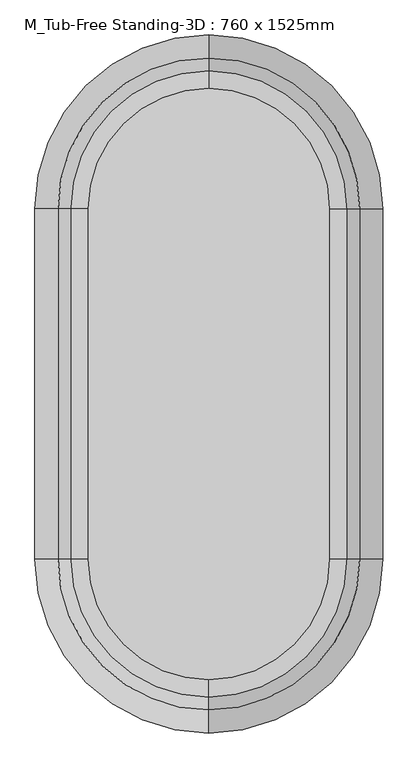
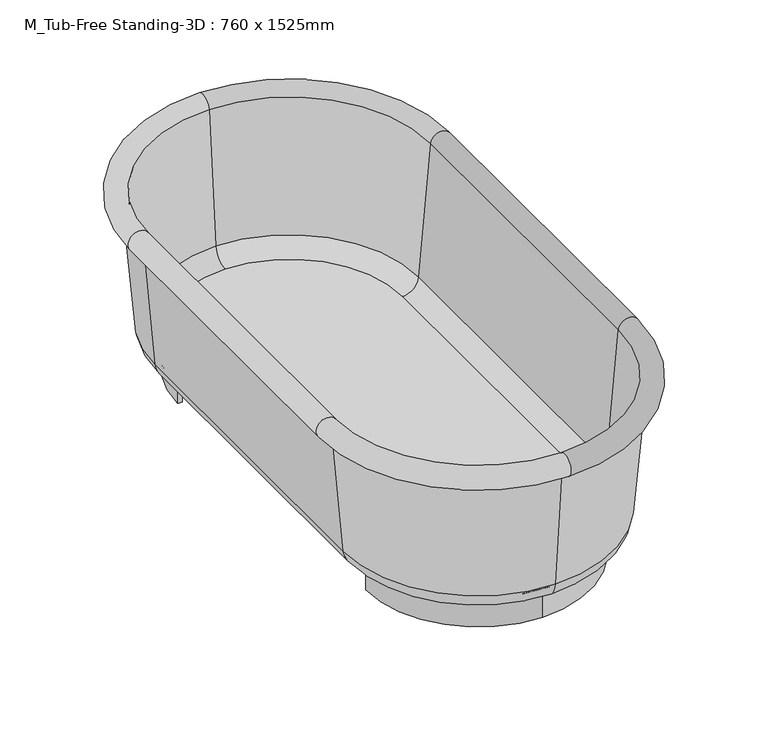
"""IFC4 building model written with IfcOpenShell, lengths in millimetres: flow terminal geometry, M_Tub-Free Standing-3D : 760 x 1525mm."""

from ifc_helpers import new_model, si_unit, point, frame, frame_2d, origin, origin_with_axes, place, context, project, spatial, polyline, circle_curve, ellipse_curve, trimmed, segment, composite_curve, outline, extrude, source, transform, mapped, element, save
from ifc_brep_helpers import plane_surface, cylinder_surface, revolved_surface, advanced_brep


def m_tub_free_standing_3d_760_x_1525mm_d9cb411c(model_context):
    return source(origin(), model_context, "Body", "SolidModel", [
        extrude(outline(composite_curve([segment(trimmed(circle_curve(frame_2d((0.0, -382.5)), 263.2824236), [point((0.0, -645.7824236))], [point((-263.2824236, -382.5))], False, "CARTESIAN"), True, "CONTINUOUS"), segment(polyline([(-263.2824236, -382.5), (-253.0, -382.5)]), True, "CONTINUOUS"), segment(trimmed(circle_curve(frame_2d((0.0, -382.5)), 253.0), [point((-253.0, -382.5))], [point((0.0, -635.5))], True, "CARTESIAN"), True, "CONTINUOUS"), segment(trimmed(circle_curve(frame_2d((0.0, -382.5)), 253.0), [point((0.0, -635.5))], [point((253.0, -382.5))], True, "CARTESIAN"), True, "CONTINUOUS"), segment(polyline([(253.0, -382.5), (263.2824236, -382.5)]), True, "CONTINUOUS"), segment(trimmed(circle_curve(frame_2d((0.0, -382.5)), 263.2824236), [point((263.2824236, -382.5))], [point((0.0, -645.7824236))], False, "CARTESIAN"), True, "CONTINUOUS")], self_intersect=False)), origin_with_axes(), (0.0, 0.0, 1.0), 66.3),
        advanced_brep(
        [(0.0, 635.5, 0.0), (-253.0, 382.5, 0.0), (-263.2824236, 382.5, 0.0), (0.0, 645.7824236, 0.0), (263.2824236, 382.5, 0.0), (253.0, 382.5, 0.0), (253.0, 382.5, 66.3), (0.0, 635.5, 66.3), (263.2824236, 382.5, 65.9536107), (263.2824236, 382.5, 66.3), (0.0, 645.7824236, 65.9536107), (-263.2824236, 382.5, 65.9536107), (-253.0, 382.5, 66.3), (-263.2824236, 382.5, 66.3), (-263.2824236, -382.5, 81.38125), (0.0, -645.7824236, 81.38125), (263.2824236, -382.5, 81.38125), (263.2824236, 382.5, 81.38125), (0.0, 645.7824236, 81.38125), (-263.2824236, 382.5, 81.38125), (263.2824236, -382.5, 66.3), (0.0, -645.7824236, 66.3), (-263.2824236, -382.5, 66.3), (-263.2824236, -382.5, 80.8774627), (0.0, -645.7824236, 80.8774627), (263.2824236, -382.5, 80.8774627), (263.2824236, 382.5, 80.8774627), (0.0, 645.7824236, 80.8774627), (-263.2824236, 382.5, 80.8774627), (0.0, -724.4, 409.2), (341.9, -382.5, 409.2), (354.6, -382.5, 409.2), (0.0, -737.1, 409.2), (0.0, -698.6045038, 114.3561295), (316.1045038, -382.5, 114.3561295), (0.0, -645.7824236, 65.9536107), (263.2824236, -382.5, 65.9536107), (0.0, -683.7374416, 115.6568289), (301.2374416, -382.5, 115.6568289), (0.0, -711.9561556, 438.1982063), (329.4561556, -382.5, 438.1982063), (-354.6, -382.5, 409.2), (-341.9, -382.5, 409.2), (-316.1045038, -382.5, 114.3561295), (-263.2824236, -382.5, 65.9536107), (-301.2374416, -382.5, 115.6568289), (-329.4561556, -382.5, 438.1982063), (-354.6, 382.5, 409.2), (-341.9, 382.5, 409.2), (-316.1045038, 382.5, 114.3561295), (-301.2374416, 382.5, 115.6568289), (-329.4561556, 382.5, 438.1982063), (0.0, 737.1, 409.2), (0.0, 724.4, 409.2), (0.0, 698.6045038, 114.3561295), (0.0, 683.7374416, 115.6568289), (0.0, 711.9561556, 438.1982063), (354.6, 382.5, 409.2), (341.9, 382.5, 409.2), (316.1045038, 382.5, 114.3561295), (301.2374416, 382.5, 115.6568289), (329.4561556, 382.5, 438.1982063)],
        [
            (0, 1, circle_curve(frame((0.0, 382.5, 0.0), z_axis=(0.0, 0.0, 1.0), x_axis=(1.0, 0.0, 0.0)), 253.0)),
            (1, 2),
            (2, 3, circle_curve(frame((0.0, 382.5, 0.0), z_axis=(0.0, 0.0, -1.0), x_axis=(1.0, 0.0, 0.0)), 263.2824236)),
            (3, 4, circle_curve(frame((0.0, 382.5, 0.0), z_axis=(0.0, 0.0, -1.0), x_axis=(1.0, 0.0, 0.0)), 263.2824236)),
            (4, 5),
            (5, 0, circle_curve(frame((0.0, 382.5, 0.0), z_axis=(0.0, 0.0, 1.0), x_axis=(1.0, 0.0, 0.0)), 253.0)),
            (5, 6),
            (6, 7, circle_curve(frame((0.0, 382.5, 66.3), z_axis=(0.0, 0.0, 1.0), x_axis=(1.0, 0.0, 0.0)), 253.0)),
            (7, 0),
            (4, 8),
            (8, 9),
            (9, 6),
            (3, 10),
            (10, 8, circle_curve(frame((0.0, 382.5, 65.9536107), z_axis=(0.0, 0.0, -1.0), x_axis=(1.0, 0.0, 0.0)), 263.2824236)),
            (2, 11),
            (11, 10, circle_curve(frame((0.0, 382.5, 65.9536107), z_axis=(0.0, 0.0, -1.0), x_axis=(1.0, 0.0, 0.0)), 263.2824236)),
            (1, 12),
            (12, 13),
            (13, 11),
            (7, 12, circle_curve(frame((0.0, 382.5, 66.3), z_axis=(0.0, 0.0, 1.0), x_axis=(1.0, 0.0, 0.0)), 253.0)),
            (14, 15, circle_curve(frame((0.0, -382.5, 81.38125), z_axis=(0.0, 0.0, 1.0), x_axis=(0.0, -1.0, 0.0)), 263.2824236)),
            (15, 16, circle_curve(frame((0.0, -382.5, 81.38125), z_axis=(0.0, 0.0, 1.0), x_axis=(0.0, -1.0, 0.0)), 263.2824236)),
            (16, 17),
            (17, 18, circle_curve(frame((0.0, 382.5, 81.38125), z_axis=(0.0, 0.0, 1.0), x_axis=(0.0, -1.0, 0.0)), 263.2824236)),
            (18, 19, circle_curve(frame((0.0, 382.5, 81.38125), z_axis=(0.0, 0.0, 1.0), x_axis=(0.0, -1.0, 0.0)), 263.2824236)),
            (19, 14),
            (9, 20),
            (20, 21, circle_curve(frame((0.0, -382.5, 66.3), z_axis=(0.0, 0.0, -1.0), x_axis=(1.0, 0.0, 0.0)), 263.2824236)),
            (21, 22, circle_curve(frame((0.0, -382.5, 66.3), z_axis=(0.0, 0.0, -1.0), x_axis=(0.0, -1.0, 0.0)), 263.2824236)),
            (22, 13),
            (14, 23),
            (23, 24, circle_curve(frame((0.0, -382.5, 80.8774627), z_axis=(0.0, 0.0, 1.0), x_axis=(0.0, -1.0, 0.0)), 263.2824236)),
            (24, 15),
            (24, 25, circle_curve(frame((0.0, -382.5, 80.8774627), z_axis=(0.0, 0.0, 1.0), x_axis=(0.0, -1.0, 0.0)), 263.2824236)),
            (25, 16),
            (25, 26),
            (26, 17),
            (26, 27, circle_curve(frame((0.0, 382.5, 80.8774627), z_axis=(0.0, 0.0, 1.0), x_axis=(0.0, -1.0, 0.0)), 263.2824236)),
            (27, 18),
            (27, 28, circle_curve(frame((0.0, 382.5, 80.8774627), z_axis=(0.0, 0.0, 1.0), x_axis=(0.0, -1.0, 0.0)), 263.2824236)),
            (28, 19),
            (28, 23),
            (29, 30, circle_curve(frame((0.0, -382.5, 409.2), z_axis=(0.0, 0.0, 1.0), x_axis=(1.0, 0.0, 0.0)), 341.9)),
            (30, 31),
            (31, 32, circle_curve(frame((0.0, -382.5, 409.2), z_axis=(0.0, 0.0, -1.0), x_axis=(1.0, 0.0, 0.0)), 354.6)),
            (32, 29),
            (29, 33),
            (33, 34, circle_curve(frame((0.0, -382.5, 114.3561295), z_axis=(0.0, 0.0, 1.0), x_axis=(1.0, 0.0, 0.0)), 316.1045038)),
            (34, 30),
            (33, 35, circle_curve(frame((0.0, -645.7824236, 118.9774627), z_axis=(1.0, 0.0, 0.0), x_axis=(0.0, -1.0, 0.0)), 53.023852)),
            (35, 36, circle_curve(frame((0.0, -382.5, 65.9536107), z_axis=(0.0, 0.0, 1.0), x_axis=(1.0, 0.0, 0.0)), 263.2824236)),
            (36, 34, circle_curve(frame((263.2824236, -382.5, 118.9774627), z_axis=(0.0, -1.0, 0.0), x_axis=(1.0, 0.0, 0.0)), 53.023852)),
            (35, 21),
            (20, 36),
            (37, 38, circle_curve(frame((0.0, -382.5, 115.6568289), z_axis=(0.0, 0.0, 1.0), x_axis=(1.0, 0.0, 0.0)), 301.2374416)),
            (38, 25, circle_curve(frame((263.2824236, -382.5, 118.9774627), z_axis=(0.0, 1.0, 0.0), x_axis=(1.0, 0.0, 0.0)), 38.1)),
            (24, 37, circle_curve(frame((0.0, -645.7824236, 118.9774627), z_axis=(-1.0, 0.0, 0.0), x_axis=(0.0, -1.0, 0.0)), 38.1)),
            (37, 39),
            (39, 40, circle_curve(frame((0.0, -382.5, 438.1982063), z_axis=(0.0, 0.0, 1.0), x_axis=(1.0, 0.0, 0.0)), 329.4561556)),
            (40, 38),
            (31, 40, circle_curve(frame((354.6, -382.5, 434.6), z_axis=(0.0, -1.0, 0.0), x_axis=(1.0, 0.0, 0.0)), 25.4)),
            (39, 32, circle_curve(frame((0.0, -737.1, 434.6), z_axis=(1.0, 0.0, 0.0), x_axis=(0.0, -1.0, 0.0)), 25.4)),
            (32, 41, circle_curve(frame((0.0, -382.5, 409.2), z_axis=(0.0, 0.0, -1.0), x_axis=(0.0, -1.0, 0.0)), 354.6)),
            (41, 42),
            (42, 29, circle_curve(frame((0.0, -382.5, 409.2), z_axis=(0.0, 0.0, 1.0), x_axis=(0.0, -1.0, 0.0)), 341.9)),
            (42, 43),
            (43, 33, circle_curve(frame((0.0, -382.5, 114.3561295), z_axis=(0.0, 0.0, 1.0), x_axis=(0.0, -1.0, 0.0)), 316.1045038)),
            (43, 44, circle_curve(frame((-263.2824236, -382.5, 118.9774627), z_axis=(0.0, -1.0, 0.0), x_axis=(-1.0, 0.0, 0.0)), 53.023852)),
            (44, 35, circle_curve(frame((0.0, -382.5, 65.9536107), z_axis=(0.0, 0.0, 1.0), x_axis=(0.0, -1.0, 0.0)), 263.2824236)),
            (44, 22),
            (23, 45, circle_curve(frame((-263.2824236, -382.5, 118.9774627), z_axis=(0.0, 1.0, 0.0), x_axis=(-1.0, 0.0, 0.0)), 38.1)),
            (45, 37, circle_curve(frame((0.0, -382.5, 115.6568289), z_axis=(0.0, 0.0, 1.0), x_axis=(0.0, -1.0, 0.0)), 301.2374416)),
            (45, 46),
            (46, 39, circle_curve(frame((0.0, -382.5, 438.1982063), z_axis=(0.0, 0.0, 1.0), x_axis=(0.0, -1.0, 0.0)), 329.4561556)),
            (46, 41, circle_curve(frame((-354.6, -382.5, 434.6), z_axis=(0.0, -1.0, 0.0), x_axis=(-1.0, 0.0, 0.0)), 25.4)),
            (41, 47),
            (47, 48),
            (48, 42),
            (48, 49),
            (49, 43),
            (49, 11, circle_curve(frame((-263.2824236, 382.5, 118.9774627), z_axis=(0.0, -1.0, 0.0), x_axis=(-1.0, 0.0, 0.0)), 53.023852)),
            (11, 44),
            (28, 50, circle_curve(frame((-263.2824236, 382.5, 118.9774627), z_axis=(0.0, 1.0, 0.0), x_axis=(-1.0, 0.0, 0.0)), 38.1)),
            (50, 45),
            (50, 51),
            (51, 46),
            (51, 47, circle_curve(frame((-354.6, 382.5, 434.6), z_axis=(0.0, -1.0, 0.0), x_axis=(-1.0, 0.0, 0.0)), 25.4)),
            (47, 52, circle_curve(frame((0.0, 382.5, 409.2), z_axis=(0.0, 0.0, -1.0), x_axis=(-1.0, 0.0, 0.0)), 354.6)),
            (52, 53),
            (53, 48, circle_curve(frame((0.0, 382.5, 409.2), z_axis=(0.0, 0.0, 1.0), x_axis=(-1.0, 0.0, 0.0)), 341.9)),
            (53, 54),
            (54, 49, circle_curve(frame((0.0, 382.5, 114.3561295), z_axis=(0.0, 0.0, 1.0), x_axis=(-1.0, 0.0, 0.0)), 316.1045038)),
            (54, 10, circle_curve(frame((0.0, 645.7824236, 118.9774627), z_axis=(-1.0, 0.0, 0.0), x_axis=(0.0, 1.0, 0.0)), 53.023852)),
            (27, 55, circle_curve(frame((0.0, 645.7824236, 118.9774627), z_axis=(1.0, 0.0, 0.0), x_axis=(0.0, 1.0, 0.0)), 38.1)),
            (55, 50, circle_curve(frame((0.0, 382.5, 115.6568289), z_axis=(0.0, 0.0, 1.0), x_axis=(-1.0, 0.0, 0.0)), 301.2374416)),
            (55, 56),
            (56, 51, circle_curve(frame((0.0, 382.5, 438.1982063), z_axis=(0.0, 0.0, 1.0), x_axis=(-1.0, 0.0, 0.0)), 329.4561556)),
            (56, 52, circle_curve(frame((0.0, 737.1, 434.6), z_axis=(-1.0, 0.0, 0.0), x_axis=(0.0, 1.0, 0.0)), 25.4)),
            (52, 57, circle_curve(frame((0.0, 382.5, 409.2), z_axis=(0.0, 0.0, -1.0), x_axis=(0.0, 1.0, 0.0)), 354.6)),
            (57, 58),
            (58, 53, circle_curve(frame((0.0, 382.5, 409.2), z_axis=(0.0, 0.0, 1.0), x_axis=(0.0, 1.0, 0.0)), 341.9)),
            (58, 59),
            (59, 54, circle_curve(frame((0.0, 382.5, 114.3561295), z_axis=(0.0, 0.0, 1.0), x_axis=(0.0, 1.0, 0.0)), 316.1045038)),
            (59, 8, circle_curve(frame((263.2824236, 382.5, 118.9774627), z_axis=(0.0, 1.0, 0.0), x_axis=(1.0, 0.0, 0.0)), 53.023852)),
            (26, 60, circle_curve(frame((263.2824236, 382.5, 118.9774627), z_axis=(0.0, -1.0, 0.0), x_axis=(1.0, 0.0, 0.0)), 38.1)),
            (60, 55, circle_curve(frame((0.0, 382.5, 115.6568289), z_axis=(0.0, 0.0, 1.0), x_axis=(0.0, 1.0, 0.0)), 301.2374416)),
            (60, 61),
            (61, 56, circle_curve(frame((0.0, 382.5, 438.1982063), z_axis=(0.0, 0.0, 1.0), x_axis=(0.0, 1.0, 0.0)), 329.4561556)),
            (61, 57, circle_curve(frame((354.6, 382.5, 434.6), z_axis=(0.0, 1.0, 0.0), x_axis=(1.0, 0.0, 0.0)), 25.4)),
            (30, 58),
            (57, 31),
            (34, 59),
            (36, 8),
            (38, 60),
            (40, 61),
        ],
        [
            plane_surface(frame((253.0, 382.5, 0.0), z_axis=(0.0, 0.0, -1.0), x_axis=(0.0, 1.0, 0.0))),
            revolved_surface(polyline([(253.0, 382.5, 0.0), (253.0, 382.5, 66.3)]), (0.0, 382.5, 0.0), (0.0, 0.0, -1.0)),
            plane_surface(frame((253.0, 382.5, 66.3), z_axis=(0.0, -1.0, 0.0), x_axis=(0.0, 0.0, -1.0))),
            cylinder_surface(frame((0.0, 382.5, 0.0), z_axis=(0.0, 0.0, 1.0), x_axis=(1.0, 0.0, 0.0)), 263.2824236),
            plane_surface(frame((-263.2824236, 382.5, 66.3), z_axis=(0.0, -1.0, 0.0), x_axis=(0.0, 0.0, -1.0))),
            plane_surface(frame((0.0, -645.7824236, 81.38125), z_axis=(0.0, 0.0, 1.0), x_axis=(1.0, 0.0, 0.0))),
            plane_surface(frame((0.0, -645.7824236, 66.3), z_axis=(0.0, 0.0, -1.0), x_axis=(-1.0, 0.0, 0.0))),
            cylinder_surface(frame((0.0, -382.5, 66.3), z_axis=(0.0, 0.0, 1.0), x_axis=(0.0, -1.0, 0.0)), 263.2824236),
            plane_surface(frame((263.2824236, -382.5, 81.38125), z_axis=(1.0, 0.0, 0.0), x_axis=(0.0, 0.0, -1.0))),
            cylinder_surface(frame((0.0, 382.5, 66.3), z_axis=(0.0, 0.0, 1.0), x_axis=(0.0, -1.0, 0.0)), 263.2824236),
            plane_surface(frame((-263.2824236, 382.5, 81.38125), z_axis=(-1.0, 0.0, 0.0), x_axis=(0.0, 0.0, -1.0))),
            plane_surface(frame((0.0, -382.5, 409.2), z_axis=(0.0, 0.0, -1.0), x_axis=(1.0, 0.0, 0.0))),
            revolved_surface(polyline([(341.9, -382.5, 409.2), (316.1045038, -382.5, 114.3561295)]), (0.0, -382.5, 434.6), (0.0, 0.0, -1.0)),
            revolved_surface(trimmed(ellipse_curve(frame((263.2824236, -382.5, 118.9774627), z_axis=(0.0, 1.0, 0.0), x_axis=(1.0, 0.0, 0.0)), 53.023852, 53.023852), [point((316.1045038, -382.5, 114.3561295))], [point((263.2824236, -382.5, 65.9536107))], True, "CARTESIAN"), (0.0, -382.5, 434.6), (0.0, 0.0, -1.0)),
            revolved_surface(polyline([(263.2824236, -382.5, 65.95361070000001), (263.2824236, -382.5, 66.30000000000001)]), (0.0, -382.5, 434.6), (0.0, 0.0, -1.0)),
            revolved_surface(trimmed(ellipse_curve(frame((263.2824236, -382.5, 118.9774627), z_axis=(0.0, -1.0, 0.0), x_axis=(1.0, 0.0, 0.0)), 38.1, 38.1), [point((263.2824236, -382.5, 80.8774627))], [point((301.2374416, -382.5, 115.6568289))], True, "CARTESIAN"), (0.0, -382.5, 434.6), (0.0, 0.0, -1.0)),
            revolved_surface(polyline([(301.2374416, -382.5, 115.6568289), (329.4561556, -382.5, 438.1982063)]), (0.0, -382.5, 434.6), (0.0, 0.0, -1.0)),
            revolved_surface(trimmed(ellipse_curve(frame((354.6, -382.5, 434.6), z_axis=(0.0, 1.0, 0.0), x_axis=(1.0, 0.0, 0.0)), 25.4, 25.4), [point((329.4561556, -382.5, 438.1982063))], [point((354.6, -382.5, 409.2))], True, "CARTESIAN"), (0.0, -382.5, 434.6), (0.0, 0.0, -1.0)),
            plane_surface(frame((0.0, -382.5, 409.2), z_axis=(0.0, 0.0, -1.0), x_axis=(0.0, -1.0, 0.0))),
            revolved_surface(polyline([(0.0, -724.4, 409.2), (0.0, -698.6045038, 114.3561295)]), (0.0, -382.5, 434.6), (0.0, 0.0, -1.0)),
            revolved_surface(trimmed(ellipse_curve(frame((0.0, -645.7824236, 118.9774627), z_axis=(1.0, 0.0, 0.0), x_axis=(0.0, -1.0, 0.0)), 53.023852, 53.023852), [point((0.0, -698.6045038, 114.3561295))], [point((0.0, -645.7824236, 65.9536107))], True, "CARTESIAN"), (0.0, -382.5, 434.6), (0.0, 0.0, -1.0)),
            revolved_surface(polyline([(0.0, -645.7824236, 65.95361070000001), (0.0, -645.7824236, 66.30000000000001)]), (0.0, -382.5, 434.6), (0.0, 0.0, -1.0)),
            revolved_surface(trimmed(ellipse_curve(frame((0.0, -645.7824236, 118.9774627), z_axis=(-1.0, 0.0, 0.0), x_axis=(0.0, -1.0, 0.0)), 38.1, 38.1), [point((0.0, -645.7824236, 80.8774627))], [point((0.0, -683.7374416, 115.6568289))], True, "CARTESIAN"), (0.0, -382.5, 434.6), (0.0, 0.0, -1.0)),
            revolved_surface(polyline([(0.0, -683.7374416, 115.6568289), (0.0, -711.9561556, 438.1982063)]), (0.0, -382.5, 434.6), (0.0, 0.0, -1.0)),
            revolved_surface(trimmed(ellipse_curve(frame((0.0, -737.1, 434.6), z_axis=(1.0, 0.0, 0.0), x_axis=(0.0, -1.0, 0.0)), 25.4, 25.4), [point((0.0, -711.9561556, 438.1982063))], [point((0.0, -737.1, 409.2))], True, "CARTESIAN"), (0.0, -382.5, 434.6), (0.0, 0.0, -1.0)),
            plane_surface(frame((-354.6, -382.5, 409.2), z_axis=(0.0, 0.0, -1.0), x_axis=(0.0, 1.0, 0.0))),
            plane_surface(frame((-341.9, -382.5, 409.2), z_axis=(-0.9961946980917455, 0.0, -0.08715574274765885), x_axis=(0.0, 1.0, 0.0))),
            cylinder_surface(frame((-263.2824236, -382.5, 118.9774627), z_axis=(0.0, -1.0, 0.0), x_axis=(-1.0, 0.0, 0.0)), 53.023852),
            plane_surface(frame((-263.2824236, -382.5, 65.9536107), z_axis=(1.0, 0.0, 0.0), x_axis=(0.0, 1.0, 0.0))),
            revolved_surface(polyline([(-301.38242360000004, 382.5, 118.9774627), (-301.38242360000004, -382.5, 118.9774627)]), (-263.2824236, -382.5, 118.9774627), (0.0, 1.0, 0.0)),
            plane_surface(frame((-301.2374416, -382.5, 115.6568289), z_axis=(0.9961946980917458, 0.0, 0.08715574274765656), x_axis=(0.0, 1.0, 0.0))),
            cylinder_surface(frame((-354.6, -382.5, 434.6), z_axis=(0.0, -1.0, 0.0), x_axis=(-1.0, 0.0, 0.0)), 25.4),
            plane_surface(frame((0.0, 382.5, 409.2), z_axis=(0.0, 0.0, -1.0), x_axis=(-1.0, 0.0, 0.0))),
            revolved_surface(polyline([(-341.9, 382.5, 409.2), (-316.1045038, 382.5, 114.3561295)]), (0.0, 382.5, 434.6), (0.0, 0.0, -1.0)),
            revolved_surface(trimmed(ellipse_curve(frame((-263.2824236, 382.5, 118.9774627), z_axis=(0.0, -1.0, 0.0), x_axis=(-1.0, 0.0, 0.0)), 53.023852, 53.023852), [point((-316.1045038, 382.5, 114.3561295))], [point((-263.2824236, 382.5, 65.9536107))], True, "CARTESIAN"), (0.0, 382.5, 434.6), (0.0, 0.0, -1.0)),
            revolved_surface(trimmed(ellipse_curve(frame((-263.2824236, 382.5, 118.9774627), z_axis=(0.0, 1.0, 0.0), x_axis=(-1.0, 0.0, 0.0)), 38.1, 38.1), [point((-263.2824236, 382.5, 80.8774627))], [point((-301.2374416, 382.5, 115.6568289))], True, "CARTESIAN"), (0.0, 382.5, 434.6), (0.0, 0.0, -1.0)),
            revolved_surface(polyline([(-301.2374416, 382.5, 115.6568289), (-329.4561556, 382.5, 438.1982063)]), (0.0, 382.5, 434.6), (0.0, 0.0, -1.0)),
            revolved_surface(trimmed(ellipse_curve(frame((-354.6, 382.5, 434.6), z_axis=(0.0, -1.0, 0.0), x_axis=(-1.0, 0.0, 0.0)), 25.4, 25.4), [point((-329.4561556, 382.5, 438.1982063))], [point((-354.6, 382.5, 409.2))], True, "CARTESIAN"), (0.0, 382.5, 434.6), (0.0, 0.0, -1.0)),
            plane_surface(frame((0.0, 382.5, 409.2), z_axis=(0.0, 0.0, -1.0), x_axis=(0.0, 1.0, 0.0))),
            revolved_surface(polyline([(0.0, 724.4, 409.2), (0.0, 698.6045038, 114.3561295)]), (0.0, 382.5, 434.6), (0.0, 0.0, -1.0)),
            revolved_surface(trimmed(ellipse_curve(frame((0.0, 645.7824236, 118.9774627), z_axis=(-1.0, 0.0, 0.0), x_axis=(0.0, 1.0, 0.0)), 53.023852, 53.023852), [point((0.0, 698.6045038, 114.3561295))], [point((0.0, 645.7824236, 65.9536107))], True, "CARTESIAN"), (0.0, 382.5, 434.6), (0.0, 0.0, -1.0)),
            revolved_surface(trimmed(ellipse_curve(frame((0.0, 645.7824236, 118.9774627), z_axis=(1.0, 0.0, 0.0), x_axis=(0.0, 1.0, 0.0)), 38.1, 38.1), [point((0.0, 645.7824236, 80.8774627))], [point((0.0, 683.7374416, 115.6568289))], True, "CARTESIAN"), (0.0, 382.5, 434.6), (0.0, 0.0, -1.0)),
            revolved_surface(polyline([(0.0, 683.7374416, 115.6568289), (0.0, 711.9561556, 438.1982063)]), (0.0, 382.5, 434.6), (0.0, 0.0, -1.0)),
            revolved_surface(trimmed(ellipse_curve(frame((0.0, 737.1, 434.6), z_axis=(-1.0, 0.0, 0.0), x_axis=(0.0, 1.0, 0.0)), 25.4, 25.4), [point((0.0, 711.9561556, 438.1982063))], [point((0.0, 737.1, 409.2))], True, "CARTESIAN"), (0.0, 382.5, 434.6), (0.0, 0.0, -1.0)),
            plane_surface(frame((354.6, 382.5, 409.2), z_axis=(0.0, 0.0, -1.0), x_axis=(0.0, -1.0, 0.0))),
            plane_surface(frame((341.9, 382.5, 409.2), z_axis=(0.9961946980917455, 0.0, -0.08715574274765885), x_axis=(0.0, -1.0, 0.0))),
            cylinder_surface(frame((263.2824236, 382.5, 118.9774627), z_axis=(0.0, 1.0, 0.0), x_axis=(1.0, 0.0, 0.0)), 53.023852),
            plane_surface(frame((263.2824236, 382.5, 65.9536107), z_axis=(-1.0, 0.0, 0.0), x_axis=(0.0, -1.0, 0.0))),
            revolved_surface(polyline([(301.38242360000004, -382.5, 118.9774627), (301.38242360000004, 382.5, 118.9774627)]), (263.2824236, 382.5, 118.9774627), (0.0, -1.0, 0.0)),
            plane_surface(frame((301.2374416, 382.5, 115.6568289), z_axis=(-0.9961946980917458, 0.0, 0.08715574274765656), x_axis=(0.0, -1.0, 0.0))),
            cylinder_surface(frame((354.6, 382.5, 434.6), z_axis=(0.0, 1.0, 0.0), x_axis=(1.0, 0.0, 0.0)), 25.4),
        ],
        [
            (0, [[1, 2, 3, 4, 5, 6]]),
            (1, [[-6, 7, 8, 9]]),
            (2, [[-5, 10, 11, 12, -7]]),
            (3, [[-4, 13, 14, -10]]),
            (3, [[-3, 15, 16, -13]]),
            (4, [[-2, 17, 18, 19, -15]]),
            (1, [[-1, -9, 20, -17]]),
            (5, [[21, 22, 23, 24, 25, 26]]),
            (6, [[-8, -12, 27, 28, 29, 30, -18, -20]]),
            (7, [[-21, 31, 32, 33]]),
            (7, [[-22, -33, 34, 35]]),
            (8, [[-23, -35, 36, 37]]),
            (9, [[-24, -37, 38, 39]]),
            (9, [[-25, -39, 40, 41]]),
            (10, [[-26, -41, 42, -31]]),
            (11, [[43, 44, 45, 46]]),
            (12, [[-43, 47, 48, 49]]),
            (13, [[-48, 50, 51, 52]]),
            (14, [[-51, 53, -28, 54]]),
            (15, [[55, 56, -34, 57]]),
            (16, [[-55, 58, 59, 60]]),
            (17, [[-45, 61, -59, 62]]),
            (18, [[-46, 63, 64, 65]]),
            (19, [[-47, -65, 66, 67]]),
            (20, [[-50, -67, 68, 69]]),
            (21, [[-69, 70, -29, -53]]),
            (22, [[-57, -32, 71, 72]]),
            (23, [[-58, -72, 73, 74]]),
            (24, [[-62, -74, 75, -63]]),
            (25, [[-64, 76, 77, 78]]),
            (26, [[-66, -78, 79, 80]]),
            (27, [[-68, -80, 81, 82]]),
            (28, [[-82, -19, -30, -70]]),
            (29, [[-71, -42, 83, 84]]),
            (30, [[-73, -84, 85, 86]]),
            (31, [[-75, -86, 87, -76]]),
            (32, [[-77, 88, 89, 90]]),
            (33, [[-79, -90, 91, 92]]),
            (34, [[-81, -92, 93, -16]]),
            (35, [[-83, -40, 94, 95]]),
            (36, [[-85, -95, 96, 97]]),
            (37, [[-87, -97, 98, -88]]),
            (38, [[-89, 99, 100, 101]]),
            (39, [[-91, -101, 102, 103]]),
            (40, [[-93, -103, 104, -14]]),
            (41, [[-94, -38, 105, 106]]),
            (42, [[-96, -106, 107, 108]]),
            (43, [[-98, -108, 109, -99]]),
            (44, [[-44, 110, -100, 111]]),
            (45, [[-49, 112, -102, -110]]),
            (46, [[-52, 113, -104, -112]]),
            (47, [[-113, -54, -27, -11]]),
            (48, [[-56, 114, -105, -36]]),
            (49, [[-60, 115, -107, -114]]),
            (50, [[-61, -111, -109, -115]]),
        ],
    ),
    ])


if __name__ == "__main__":
    model = new_model("IFC4")
    model_context = context("Model", 3, world=origin())
    ifc_project = project(units=[si_unit("LENGTHUNIT", "METRE", prefix="MILLI")], contexts=[model_context])
    site = spatial("IfcSite", under=ifc_project)
    building = spatial("IfcBuilding", under=site)
    placement = place(None, origin())
    m_tub_free_standing_3d_760_x_1525mm_shape = m_tub_free_standing_3d_760_x_1525mm_d9cb411c(model_context)
    element("IfcFlowTerminal", 1, ObjectType="M_Tub-Free Standing-3D : 760 x 1525mm", at=placement, inside=building, context=model_context, shape_type="MappedRepresentation", body=[
        mapped(m_tub_free_standing_3d_760_x_1525mm_shape, transform((0.0, 0.0, 0.0), x_axis=(1.0, 0.0, 0.0), y_axis=(0.0, 1.0, 0.0), z_axis=(0.0, 0.0, 1.0))),
    ])
    save(model, "model.ifc")

# Revit data of these elements
# Type "M_Tub-Free Standing-3D : 760 x 1525mm"
#   Height = 460 mm
#   Length = 1525 mm
#   Width = 760 mm
#   Tub Material = Porcelain, Ivory
#   Default Elevation = 0
# Element 1 (IfcFlowTerminal, "M_Tub-Free Standing-3D : 760 x 1525mm")
#   Materials on its faces: "Porcelain, Ivory"
# Materials
#   "Porcelain, Ivory": class "Ceramic", colour RGB 247 247 239, transparency 0, Description = "Porcelain, ivory", Cost = 0
